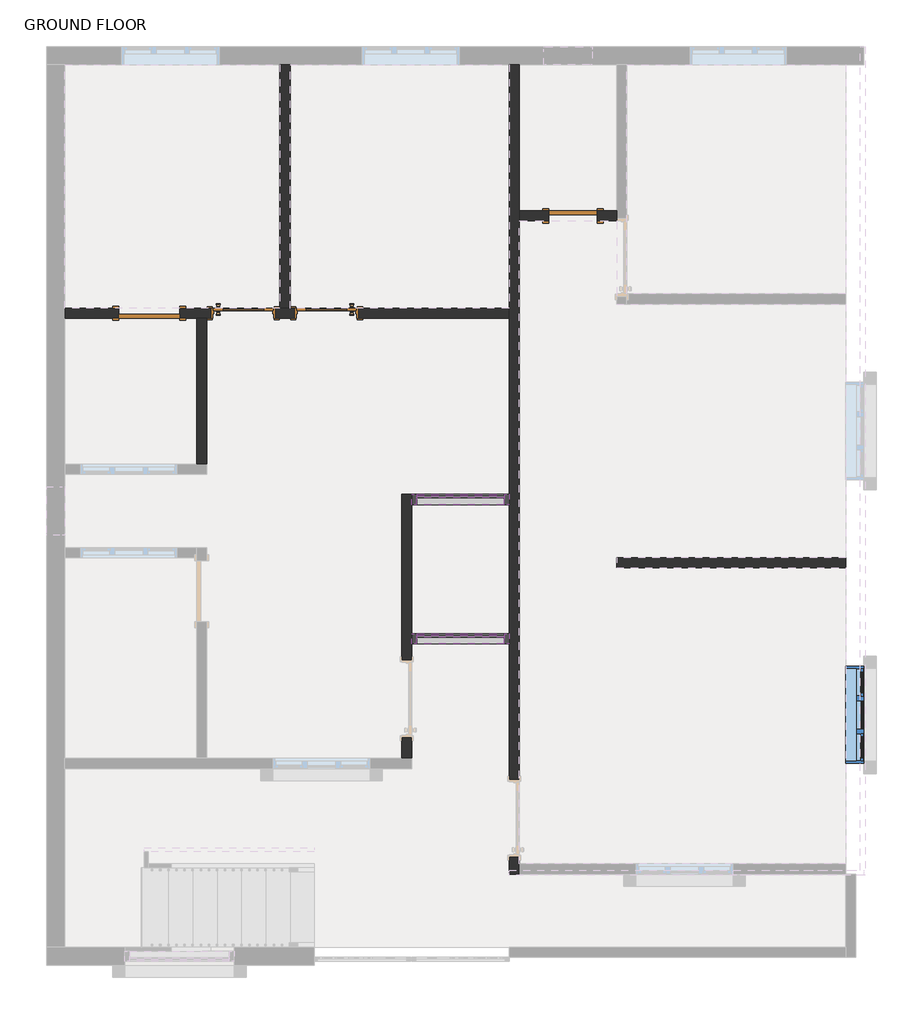
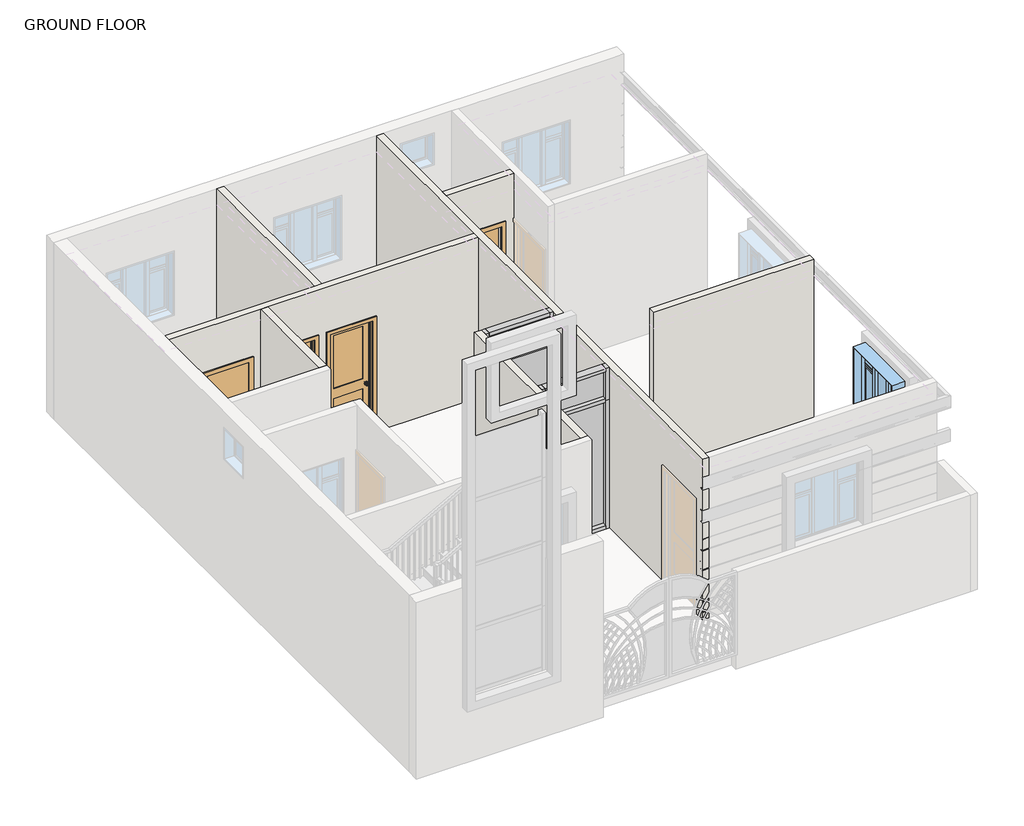
# One storey, part 3 of 7: 14 members, 7 walls, 4 doors, 4 plates, 1 window.
"""IFC4 building model written with IfcOpenShell, lengths in millimetres."""

from ifc_helpers import new_model, si_unit, frame, origin, place, context, project, spatial, polyline, circle_curve, outline, extrude, faceted_brep, transform, mapped, element, save
from ifc_brep_helpers import plane_surface, cylinder_surface, revolved_surface, advanced_brep
from components import door_interior_single_2_panel_wood_main_doors_a5f98f63, door_interior_single_2_panel_wood_main_doors_4d656947, single_flush_bathroom_flush_door_4d6c7550, single_flush_bathroom_flush_door_2_931cabab, member_273a15f2, member_867fe1e1, member_ee409385, member_47bfaf8a, system_panel_glazed_c5a9eb28, system_panel_glazed_3290db12, window_casement_triple_side_transom_window_4_x_4_fd24aed3

model = new_model("IFC4")

# Units and contexts
model_context = context("Model", 3, world=origin())
ifc_project = project(units=[si_unit("LENGTHUNIT", "METRE", prefix="MILLI")], contexts=[model_context])

# Site, building, storey
site = spatial("IfcSite", under=ifc_project)
building = spatial("IfcBuilding", under=site)
storey = spatial("IfcBuildingStorey", under=building, Name="GROUND FLOOR", Elevation=304.8)

# Doors
placement = place(None, origin())
door_interior_single_2_panel_wood_main_doors_shape = door_interior_single_2_panel_wood_main_doors_a5f98f63(model_context)
element("IfcDoor", 1, ObjectType="Door-Interior-Single-2_Panel-Wood : MAIN DOORS", at=placement, inside=storey, context=model_context, shape_type="MappedRepresentation", body=[
    mapped(door_interior_single_2_panel_wood_main_doors_shape, transform((-12525.5023867, 5183.9250137, 304.8), x_axis=(1.0, 0.0, 0.0), y_axis=(0.0, 1.0, 0.0), z_axis=(0.0, 0.0, 1.0))),
])
door_interior_single_2_panel_wood_main_doors_2_shape = door_interior_single_2_panel_wood_main_doors_4d656947(model_context)
element("IfcDoor", 2, ObjectType="Door-Interior-Single-2_Panel-Wood : MAIN DOORS", at=placement, inside=storey, context=model_context, shape_type="MappedRepresentation", body=[
    mapped(door_interior_single_2_panel_wood_main_doors_2_shape, transform((-11484.1023867, 5183.9250137, 304.8), x_axis=(-1.0, 0.0, 0.0), y_axis=(0.0, -1.0, 0.0), z_axis=(0.0, 0.0, 1.0))),
])
single_flush_bathroom_flush_door_shape = single_flush_bathroom_flush_door_4d6c7550(model_context)
element("IfcDoor", 3, ObjectType="Single-Flush : BATHROOM FLUSH DOOR", at=placement, inside=storey, context=model_context, shape_type="MappedRepresentation", body=[
    mapped(single_flush_bathroom_flush_door_shape, transform((-13706.6023867, 5180.7500137, 304.8), x_axis=(-1.0, 0.0, 0.0), y_axis=(0.0, -1.0, 0.0), z_axis=(0.0, 0.0, 1.0))),
])
single_flush_bathroom_flush_door_2_shape = single_flush_bathroom_flush_door_2_931cabab(model_context)
element("IfcDoor", 4, ObjectType="Single-Flush : BATHROOM FLUSH DOOR 2", at=placement, inside=storey, context=model_context, shape_type="MappedRepresentation", body=[
    mapped(single_flush_bathroom_flush_door_2_shape, transform((-8398.0023867, 6399.9500137, 304.8), x_axis=(-1.0, 0.0, 0.0), y_axis=(0.0, -1.0, 0.0), z_axis=(0.0, 0.0, 1.0))),
])

# Members
member_shape = member_273a15f2(model_context)
element("IfcMember", 5, ObjectType="Rectangular Mullion : 2.5\" x 5\" rectangular", at=placement, inside=storey, context=model_context, shape_type="MappedRepresentation", body=[
    mapped(member_shape, transform((-9261.6023867, 2848.1833471, 3352.8), x_axis=(0.0, 0.0, 1.0), y_axis=(0.0, -1.0, 0.0), z_axis=(1.0, 0.0, 0.0))),
])
element("IfcMember", 6, ObjectType="Rectangular Mullion : 2.5\" x 5\" rectangular", at=placement, inside=storey, context=model_context, shape_type="MappedRepresentation", body=[
    mapped(member_shape, transform((-9261.6023867, 1104.0500137, 3352.8), x_axis=(0.0, 0.0, 1.0), y_axis=(0.0, -1.0, 0.0), z_axis=(1.0, 0.0, 0.0))),
])
element("IfcMember", 7, ObjectType="Rectangular Mullion : 2.5\" x 5\" rectangular", at=placement, inside=storey, context=model_context, shape_type="MappedRepresentation", body=[
    mapped(member_shape, transform((-10353.8023867, 2848.1833471, 304.8), x_axis=(0.0, 0.0, -1.0), y_axis=(0.0, -1.0, 0.0), z_axis=(-1.0, 0.0, 0.0))),
])
element("IfcMember", 8, ObjectType="Rectangular Mullion : 2.5\" x 5\" rectangular", at=placement, inside=storey, context=model_context, shape_type="MappedRepresentation", body=[
    mapped(member_shape, transform((-10353.8023867, 1104.0500137, 304.8), x_axis=(0.0, 0.0, -1.0), y_axis=(0.0, -1.0, 0.0), z_axis=(-1.0, 0.0, 0.0))),
])
member_2_shape = member_867fe1e1(model_context)
element("IfcMember", 9, ObjectType="Rectangular Mullion : 2.5\" x 5\" rectangular", at=placement, inside=storey, context=model_context, shape_type="MappedRepresentation", body=[
    mapped(member_2_shape, transform((-9261.6023867, 2848.1833471, 2743.2), x_axis=(0.0, 0.0, 1.0), y_axis=(0.0, -1.0, 0.0), z_axis=(1.0, 0.0, 0.0))),
])
element("IfcMember", 10, ObjectType="Rectangular Mullion : 2.5\" x 5\" rectangular", at=placement, inside=storey, context=model_context, shape_type="MappedRepresentation", body=[
    mapped(member_2_shape, transform((-9261.6023867, 1104.0500137, 2743.2), x_axis=(0.0, 0.0, 1.0), y_axis=(0.0, -1.0, 0.0), z_axis=(1.0, 0.0, 0.0))),
])
member_3_shape = member_ee409385(model_context)
element("IfcMember", 11, ObjectType="Rectangular Mullion : 2.5\" x 5\" rectangular", at=placement, inside=storey, context=model_context, shape_type="MappedRepresentation", body=[
    mapped(member_3_shape, transform((-9198.1023867, 2848.1833471, 304.8), x_axis=(1.0, 0.0, 0.0), y_axis=(0.0, -1.0, 0.0), z_axis=(0.0, 0.0, -1.0))),
])
element("IfcMember", 12, ObjectType="Rectangular Mullion : 2.5\" x 5\" rectangular", at=placement, inside=storey, context=model_context, shape_type="MappedRepresentation", body=[
    mapped(member_3_shape, transform((-9198.1023867, 1104.0500137, 304.8), x_axis=(1.0, 0.0, 0.0), y_axis=(0.0, -1.0, 0.0), z_axis=(0.0, 0.0, -1.0))),
])
member_4_shape = member_47bfaf8a(model_context)
element("IfcMember", 13, ObjectType="Rectangular Mullion : 2.5\" x 5\" rectangular", at=placement, inside=storey, context=model_context, shape_type="MappedRepresentation", body=[
    mapped(member_4_shape, transform((-10417.3023867, 2848.1833471, 3352.8), x_axis=(-1.0, 0.0, 0.0), y_axis=(0.0, -1.0, 0.0), z_axis=(0.0, 0.0, 1.0))),
])
element("IfcMember", 14, ObjectType="Rectangular Mullion : 2.5\" x 5\" rectangular", at=placement, inside=storey, context=model_context, shape_type="MappedRepresentation", body=[
    mapped(member_4_shape, transform((-10417.3023867, 1104.0500137, 3352.8), x_axis=(-1.0, 0.0, 0.0), y_axis=(0.0, -1.0, 0.0), z_axis=(0.0, 0.0, 1.0))),
])
element("IfcMember", 15, ObjectType="Rectangular Mullion : 2.5\" x 5\" rectangular", at=placement, inside=storey, context=model_context, shape_type="MappedRepresentation", body=[
    mapped(member_4_shape, transform((-9198.1023867, 2848.1833471, 2743.2), x_axis=(1.0, 0.0, 0.0), y_axis=(0.0, -1.0, 0.0), z_axis=(0.0, 0.0, -1.0))),
])
element("IfcMember", 16, ObjectType="Rectangular Mullion : 2.5\" x 5\" rectangular", at=placement, inside=storey, context=model_context, shape_type="MappedRepresentation", body=[
    mapped(member_4_shape, transform((-9198.1023867, 1104.0500137, 2743.2), x_axis=(1.0, 0.0, 0.0), y_axis=(0.0, -1.0, 0.0), z_axis=(0.0, 0.0, -1.0))),
])
element("IfcMember", 17, ObjectType="Rectangular Mullion : 2.5\" x 5\" rectangular", at=placement, inside=storey, context=model_context, shape_type="MappedRepresentation", body=[
    mapped(member_3_shape, transform((-10417.3023867, 2848.1833471, 2743.2), x_axis=(-1.0, 0.0, 0.0), y_axis=(0.0, -1.0, 0.0), z_axis=(0.0, 0.0, 1.0))),
])
element("IfcMember", 18, ObjectType="Rectangular Mullion : 2.5\" x 5\" rectangular", at=placement, inside=storey, context=model_context, shape_type="MappedRepresentation", body=[
    mapped(member_3_shape, transform((-10417.3023867, 1104.0500137, 2743.2), x_axis=(-1.0, 0.0, 0.0), y_axis=(0.0, -1.0, 0.0), z_axis=(0.0, 0.0, 1.0))),
])

# Plates
system_panel_glazed_shape = system_panel_glazed_c5a9eb28(model_context)
element("IfcPlate", 19, ObjectType="System Panel : Glazed", at=placement, inside=storey, context=model_context, shape_type="MappedRepresentation", body=[
    mapped(system_panel_glazed_shape, transform((-9807.7023867, 2848.1833471, 368.3), x_axis=(1.0, 0.0, 0.0), y_axis=(0.0, 1.0, 0.0), z_axis=(0.0, 0.0, 1.0))),
])
element("IfcPlate", 20, ObjectType="System Panel : Glazed", at=placement, inside=storey, context=model_context, shape_type="MappedRepresentation", body=[
    mapped(system_panel_glazed_shape, transform((-9807.7023867, 1104.0500137, 368.3), x_axis=(1.0, 0.0, 0.0), y_axis=(0.0, 1.0, 0.0), z_axis=(0.0, 0.0, 1.0))),
])
system_panel_glazed_2_shape = system_panel_glazed_3290db12(model_context)
element("IfcPlate", 21, ObjectType="System Panel : Glazed", at=placement, inside=storey, context=model_context, shape_type="MappedRepresentation", body=[
    mapped(system_panel_glazed_2_shape, transform((-9807.7023867, 2848.1833471, 2774.95), x_axis=(1.0, 0.0, 0.0), y_axis=(0.0, 1.0, 0.0), z_axis=(0.0, 0.0, 1.0))),
])
element("IfcPlate", 22, ObjectType="System Panel : Glazed", at=placement, inside=storey, context=model_context, shape_type="MappedRepresentation", body=[
    mapped(system_panel_glazed_2_shape, transform((-9807.7023867, 1104.0500137, 2774.95), x_axis=(1.0, 0.0, 0.0), y_axis=(0.0, 1.0, 0.0), z_axis=(0.0, 0.0, 1.0))),
])

# Walls
element("IfcWall", 23, ObjectType="INNER WALL 5\"", at=placement, inside=storey, context=model_context, shape_type="AdvancedBrep", body=[
    advanced_brep(
    [(-9198.1023867, -1842.3499863, 3352.8), (-9198.1023867, 5117.2500137, 3352.8), (-9198.1023867, 5244.2500137, 3352.8), (-9198.1023867, 8292.2500137, 3352.8), (-9198.1023867, 8292.2500137, 304.8), (-9198.1023867, 5244.2500137, 304.8), (-9198.1023867, 5117.2500137, 304.8), (-9198.1023867, -661.2499863, 304.8), (-9198.1023867, -661.2499863, 2463.8), (-9198.1023867, -1626.4499863, 2463.8), (-9198.1023867, -1626.4499863, 304.8), (-9198.1023867, -1842.3499863, 304.8), (-9198.1023867, -1842.3499863, 444.5), (-9198.1023867, -1793.9883863, 444.5), (-9198.1023867, -1793.9883863, 445.8796758), (-9198.1023867, -1798.3711955, 451.0534103), (-9198.1023867, -1821.9918863, 454.9902), (-9198.1023867, -1841.2297679, 458.19652), (-9198.1023867, -1842.3499863, 458.44689), (-9198.1023867, -1842.3499863, 659.15311), (-9198.1023867, -1841.2297679, 659.40348), (-9198.1023867, -1821.9918863, 662.6098), (-9198.1023867, -1798.3711955, 666.5465897), (-9198.1023867, -1793.9883863, 671.7203242), (-9198.1023867, -1793.9883863, 673.1), (-9198.1023867, -1842.3499863, 673.1), (-9198.1023867, -1842.3499863, 1028.7), (-9198.1023867, -1793.9883863, 1028.7), (-9198.1023867, -1793.9883863, 1030.0796758), (-9198.1023867, -1798.3711955, 1035.2534103), (-9198.1023867, -1821.9918863, 1039.1902), (-9198.1023867, -1841.2297679, 1042.39652), (-9198.1023867, -1842.3499863, 1042.64689), (-9198.1023867, -1842.3499863, 1243.35311), (-9198.1023867, -1841.2297679, 1243.60348), (-9198.1023867, -1821.9918863, 1246.8098), (-9198.1023867, -1798.3711955, 1250.7465897), (-9198.1023867, -1793.9883863, 1255.9203242), (-9198.1023867, -1793.9883863, 1257.3), (-9198.1023867, -1842.3499863, 1257.3), (-9198.1023867, -1842.3499863, 1612.9), (-9198.1023867, -1793.9883863, 1612.9), (-9198.1023867, -1793.9883863, 1614.2796758), (-9198.1023867, -1798.3711955, 1619.4534103), (-9198.1023867, -1821.9918863, 1623.3902), (-9198.1023867, -1841.2297679, 1626.59652), (-9198.1023867, -1842.3499863, 1626.84689), (-9198.1023867, -1842.3499863, 1827.55311), (-9198.1023867, -1841.2297679, 1827.80348), (-9198.1023867, -1821.9918863, 1831.0098), (-9198.1023867, -1798.3711955, 1834.9465897), (-9198.1023867, -1793.9883863, 1840.1203242), (-9198.1023867, -1793.9883863, 1841.5), (-9198.1023867, -1842.3499863, 1841.5), (-9198.1023867, -1842.3499863, 2146.3), (-9198.1023867, -1793.9883863, 2146.3), (-9198.1023867, -1793.9883863, 2147.6796758), (-9198.1023867, -1798.3711955, 2152.8534103), (-9198.1023867, -1821.9918863, 2156.7902), (-9198.1023867, -1841.2297679, 2159.99652), (-9198.1023867, -1842.3499863, 2160.24689), (-9198.1023867, -1842.3499863, 2360.95311), (-9198.1023867, -1841.2297679, 2361.20348), (-9198.1023867, -1821.9918863, 2364.4098), (-9198.1023867, -1798.3711955, 2368.3465897), (-9198.1023867, -1793.9883863, 2373.5203242), (-9198.1023867, -1793.9883863, 2374.9), (-9198.1023867, -1842.3499863, 2374.9), (-9198.1023867, -1842.3499863, 2781.3), (-9198.1023867, -1793.9883863, 2781.3), (-9198.1023867, -1793.9883863, 2782.6796758), (-9198.1023867, -1798.3711955, 2787.8534103), (-9198.1023867, -1821.9918863, 2791.7902), (-9198.1023867, -1841.2297679, 2794.99652), (-9198.1023867, -1842.3499863, 2795.24689), (-9198.1023867, -1842.3499863, 2995.95311), (-9198.1023867, -1841.2297679, 2996.20348), (-9198.1023867, -1821.9918863, 2999.4098), (-9198.1023867, -1798.3711955, 3003.3465897), (-9198.1023867, -1793.9883863, 3008.5203242), (-9198.1023867, -1793.9883863, 3009.9), (-9198.1023867, -1842.3499863, 3009.9), (-9071.1023867, 8292.2500137, 3352.8), (-9071.1023867, 6463.4500137, 3352.8), (-9071.1023867, 6336.4500137, 3352.8), (-9071.1023867, -1715.3499863, 3352.8), (-9071.1023867, -1842.3499863, 3352.8), (-9071.1023867, -1842.3499863, 3009.9), (-9071.1023867, -1793.9883863, 3009.9), (-9071.1023867, -1793.9883863, 3008.5203242), (-9071.1023867, -1798.3711955, 3003.3465897), (-9071.1023867, -1821.9918863, 2999.4098), (-9071.1023867, -1841.2297679, 2996.20348), (-9071.1023867, -1842.3499863, 2995.95311), (-9071.1023867, -1842.3499863, 2795.24689), (-9071.1023867, -1841.2297679, 2794.99652), (-9071.1023867, -1821.9918863, 2791.7902), (-9071.1023867, -1798.3711955, 2787.8534103), (-9071.1023867, -1793.9883863, 2782.6796758), (-9071.1023867, -1793.9883863, 2781.3), (-9071.1023867, -1842.3499863, 2781.3), (-9071.1023867, -1842.3499863, 2374.9), (-9071.1023867, -1793.9883863, 2374.9), (-9071.1023867, -1793.9883863, 2373.5203242), (-9071.1023867, -1798.3711955, 2368.3465897), (-9071.1023867, -1821.9918863, 2364.4098), (-9071.1023867, -1841.2297679, 2361.20348), (-9071.1023867, -1842.3499863, 2360.95311), (-9071.1023867, -1842.3499863, 2160.24689), (-9071.1023867, -1841.2297679, 2159.99652), (-9071.1023867, -1821.9918863, 2156.7902), (-9071.1023867, -1798.3711955, 2152.8534103), (-9071.1023867, -1793.9883863, 2147.6796758), (-9071.1023867, -1793.9883863, 2146.3), (-9071.1023867, -1842.3499863, 2146.3), (-9071.1023867, -1842.3499863, 1841.5), (-9071.1023867, -1793.9883863, 1841.5), (-9071.1023867, -1793.9883863, 1840.1203242), (-9071.1023867, -1798.3711955, 1834.9465897), (-9071.1023867, -1821.9918863, 1831.0098), (-9071.1023867, -1841.2297679, 1827.80348), (-9071.1023867, -1842.3499863, 1827.55311), (-9071.1023867, -1842.3499863, 1626.84689), (-9071.1023867, -1841.2297679, 1626.59652), (-9071.1023867, -1821.9918863, 1623.3902), (-9071.1023867, -1798.3711955, 1619.4534103), (-9071.1023867, -1793.9883863, 1614.2796758), (-9071.1023867, -1793.9883863, 1612.9), (-9071.1023867, -1842.3499863, 1612.9), (-9071.1023867, -1842.3499863, 1257.3), (-9071.1023867, -1793.9883863, 1257.3), (-9071.1023867, -1793.9883863, 1255.9203242), (-9071.1023867, -1798.3711955, 1250.7465897), (-9071.1023867, -1821.9918863, 1246.8098), (-9071.1023867, -1841.2297679, 1243.60348), (-9071.1023867, -1842.3499863, 1243.35311), (-9071.1023867, -1842.3499863, 1042.64689), (-9071.1023867, -1841.2297679, 1042.39652), (-9071.1023867, -1821.9918863, 1039.1902), (-9071.1023867, -1798.3711955, 1035.2534103), (-9071.1023867, -1793.9883863, 1030.0796758), (-9071.1023867, -1793.9883863, 1028.7), (-9071.1023867, -1842.3499863, 1028.7), (-9071.1023867, -1842.3499863, 673.1), (-9071.1023867, -1793.9883863, 673.1), (-9071.1023867, -1793.9883863, 671.7203242), (-9071.1023867, -1798.3711955, 666.5465897), (-9071.1023867, -1821.9918863, 662.6098), (-9071.1023867, -1841.2297679, 659.40348), (-9071.1023867, -1842.3499863, 659.15311), (-9071.1023867, -1842.3499863, 458.44689), (-9071.1023867, -1841.2297679, 458.19652), (-9071.1023867, -1821.9918863, 454.9902), (-9071.1023867, -1798.3711955, 451.0534103), (-9071.1023867, -1793.9883863, 445.8796758), (-9071.1023867, -1793.9883863, 444.5), (-9071.1023867, -1842.3499863, 444.5), (-9071.1023867, -1842.3499863, 304.8), (-9071.1023867, -1626.4499863, 304.8), (-9071.1023867, -1626.4499863, 2463.8), (-9071.1023867, -661.2499863, 2463.8), (-9071.1023867, -661.2499863, 304.8), (-9071.1023867, 6336.4500137, 304.8), (-9071.1023867, 6463.4500137, 304.8), (-9071.1023867, 8292.2500137, 304.8)],
    [
        (0, 1),
        (1, 2),
        (2, 3),
        (3, 4),
        (4, 5),
        (5, 6),
        (6, 7),
        (7, 8),
        (8, 9),
        (9, 10),
        (10, 11),
        (11, 12),
        (12, 13),
        (13, 14),
        (14, 15, circle_curve(frame((-9198.1023867, -1799.2334863, 445.8796758), z_axis=(1.0, 0.0, 0.0), x_axis=(0.0, 1.0, 0.0)), 5.2451)),
        (15, 16),
        (16, 17),
        (17, 18, circle_curve(frame((-9198.1023867, -1839.5051863, 468.543989), z_axis=(-1.0, 0.0, 0.0), x_axis=(0.0, 1.0, 0.0)), 10.4902)),
        (18, 19),
        (19, 20, circle_curve(frame((-9198.1023867, -1839.5051863, 649.056011), z_axis=(-1.0, 0.0, 0.0), x_axis=(0.0, 1.0, 0.0)), 10.4902)),
        (20, 21),
        (21, 22),
        (22, 23, circle_curve(frame((-9198.1023867, -1799.2334863, 671.7203242), z_axis=(1.0, 0.0, 0.0), x_axis=(0.0, 1.0, 0.0)), 5.2451)),
        (23, 24),
        (24, 25),
        (25, 26),
        (26, 27),
        (27, 28),
        (28, 29, circle_curve(frame((-9198.1023867, -1799.2334863, 1030.0796758), z_axis=(1.0, 0.0, 0.0), x_axis=(0.0, 1.0, 0.0)), 5.2451)),
        (29, 30),
        (30, 31),
        (31, 32, circle_curve(frame((-9198.1023867, -1839.5051863, 1052.743989), z_axis=(-1.0, 0.0, 0.0), x_axis=(0.0, 1.0, 0.0)), 10.4902)),
        (32, 33),
        (33, 34, circle_curve(frame((-9198.1023867, -1839.5051863, 1233.256011), z_axis=(-1.0, 0.0, 0.0), x_axis=(0.0, 1.0, 0.0)), 10.4902)),
        (34, 35),
        (35, 36),
        (36, 37, circle_curve(frame((-9198.1023867, -1799.2334863, 1255.9203242), z_axis=(1.0, 0.0, 0.0), x_axis=(0.0, 1.0, 0.0)), 5.2451)),
        (37, 38),
        (38, 39),
        (39, 40),
        (40, 41),
        (41, 42),
        (42, 43, circle_curve(frame((-9198.1023867, -1799.2334863, 1614.2796758), z_axis=(1.0, 0.0, 0.0), x_axis=(0.0, 1.0, 0.0)), 5.2451)),
        (43, 44),
        (44, 45),
        (45, 46, circle_curve(frame((-9198.1023867, -1839.5051863, 1636.943989), z_axis=(-1.0, 0.0, 0.0), x_axis=(0.0, 1.0, 0.0)), 10.4902)),
        (46, 47),
        (47, 48, circle_curve(frame((-9198.1023867, -1839.5051863, 1817.456011), z_axis=(-1.0, 0.0, 0.0), x_axis=(0.0, 1.0, 0.0)), 10.4902)),
        (48, 49),
        (49, 50),
        (50, 51, circle_curve(frame((-9198.1023867, -1799.2334863, 1840.1203242), z_axis=(1.0, 0.0, 0.0), x_axis=(0.0, 1.0, 0.0)), 5.2451)),
        (51, 52),
        (52, 53),
        (53, 54),
        (54, 55),
        (55, 56),
        (56, 57, circle_curve(frame((-9198.1023867, -1799.2334863, 2147.6796758), z_axis=(1.0, 0.0, 0.0), x_axis=(0.0, 1.0, 0.0)), 5.2451)),
        (57, 58),
        (58, 59),
        (59, 60, circle_curve(frame((-9198.1023867, -1839.5051863, 2170.343989), z_axis=(-1.0, 0.0, 0.0), x_axis=(0.0, 1.0, 0.0)), 10.4902)),
        (60, 61),
        (61, 62, circle_curve(frame((-9198.1023867, -1839.5051863, 2350.856011), z_axis=(-1.0, 0.0, 0.0), x_axis=(0.0, 1.0, 0.0)), 10.4902)),
        (62, 63),
        (63, 64),
        (64, 65, circle_curve(frame((-9198.1023867, -1799.2334863, 2373.5203242), z_axis=(1.0, 0.0, 0.0), x_axis=(0.0, 1.0, 0.0)), 5.2451)),
        (65, 66),
        (66, 67),
        (67, 68),
        (68, 69),
        (69, 70),
        (70, 71, circle_curve(frame((-9198.1023867, -1799.2334863, 2782.6796758), z_axis=(1.0, 0.0, 0.0), x_axis=(0.0, 1.0, 0.0)), 5.2451)),
        (71, 72),
        (72, 73),
        (73, 74, circle_curve(frame((-9198.1023867, -1839.5051863, 2805.343989), z_axis=(-1.0, 0.0, 0.0), x_axis=(0.0, 1.0, 0.0)), 10.4902)),
        (74, 75),
        (75, 76, circle_curve(frame((-9198.1023867, -1839.5051863, 2985.856011), z_axis=(-1.0, 0.0, 0.0), x_axis=(0.0, 1.0, 0.0)), 10.4902)),
        (76, 77),
        (77, 78),
        (78, 79, circle_curve(frame((-9198.1023867, -1799.2334863, 3008.5203242), z_axis=(1.0, 0.0, 0.0), x_axis=(0.0, 1.0, 0.0)), 5.2451)),
        (79, 80),
        (80, 81),
        (81, 0),
        (82, 83),
        (83, 84),
        (84, 85),
        (85, 86),
        (86, 87),
        (87, 88),
        (88, 89),
        (89, 90, circle_curve(frame((-9071.1023867, -1799.2334863, 3008.5203242), z_axis=(-1.0, 0.0, 0.0), x_axis=(0.0, 1.0, 0.0)), 5.2451)),
        (90, 91),
        (91, 92),
        (92, 93, circle_curve(frame((-9071.1023867, -1839.5051863, 2985.856011), z_axis=(1.0, 0.0, 0.0), x_axis=(0.0, 1.0, 0.0)), 10.4902)),
        (93, 94),
        (94, 95, circle_curve(frame((-9071.1023867, -1839.5051863, 2805.343989), z_axis=(1.0, 0.0, 0.0), x_axis=(0.0, 1.0, 0.0)), 10.4902)),
        (95, 96),
        (96, 97),
        (97, 98, circle_curve(frame((-9071.1023867, -1799.2334863, 2782.6796758), z_axis=(-1.0, 0.0, 0.0), x_axis=(0.0, 1.0, 0.0)), 5.2451)),
        (98, 99),
        (99, 100),
        (100, 101),
        (101, 102),
        (102, 103),
        (103, 104, circle_curve(frame((-9071.1023867, -1799.2334863, 2373.5203242), z_axis=(-1.0, 0.0, 0.0), x_axis=(0.0, 1.0, 0.0)), 5.2451)),
        (104, 105),
        (105, 106),
        (106, 107, circle_curve(frame((-9071.1023867, -1839.5051863, 2350.856011), z_axis=(1.0, 0.0, 0.0), x_axis=(0.0, 1.0, 0.0)), 10.4902)),
        (107, 108),
        (108, 109, circle_curve(frame((-9071.1023867, -1839.5051863, 2170.343989), z_axis=(1.0, 0.0, 0.0), x_axis=(0.0, 1.0, 0.0)), 10.4902)),
        (109, 110),
        (110, 111),
        (111, 112, circle_curve(frame((-9071.1023867, -1799.2334863, 2147.6796758), z_axis=(-1.0, 0.0, 0.0), x_axis=(0.0, 1.0, 0.0)), 5.2451)),
        (112, 113),
        (113, 114),
        (114, 115),
        (115, 116),
        (116, 117),
        (117, 118, circle_curve(frame((-9071.1023867, -1799.2334863, 1840.1203242), z_axis=(-1.0, 0.0, 0.0), x_axis=(0.0, 1.0, 0.0)), 5.2451)),
        (118, 119),
        (119, 120),
        (120, 121, circle_curve(frame((-9071.1023867, -1839.5051863, 1817.456011), z_axis=(1.0, 0.0, 0.0), x_axis=(0.0, 1.0, 0.0)), 10.4902)),
        (121, 122),
        (122, 123, circle_curve(frame((-9071.1023867, -1839.5051863, 1636.943989), z_axis=(1.0, 0.0, 0.0), x_axis=(0.0, 1.0, 0.0)), 10.4902)),
        (123, 124),
        (124, 125),
        (125, 126, circle_curve(frame((-9071.1023867, -1799.2334863, 1614.2796758), z_axis=(-1.0, 0.0, 0.0), x_axis=(0.0, 1.0, 0.0)), 5.2451)),
        (126, 127),
        (127, 128),
        (128, 129),
        (129, 130),
        (130, 131),
        (131, 132, circle_curve(frame((-9071.1023867, -1799.2334863, 1255.9203242), z_axis=(-1.0, 0.0, 0.0), x_axis=(0.0, 1.0, 0.0)), 5.2451)),
        (132, 133),
        (133, 134),
        (134, 135, circle_curve(frame((-9071.1023867, -1839.5051863, 1233.256011), z_axis=(1.0, 0.0, 0.0), x_axis=(0.0, 1.0, 0.0)), 10.4902)),
        (135, 136),
        (136, 137, circle_curve(frame((-9071.1023867, -1839.5051863, 1052.743989), z_axis=(1.0, 0.0, 0.0), x_axis=(0.0, 1.0, 0.0)), 10.4902)),
        (137, 138),
        (138, 139),
        (139, 140, circle_curve(frame((-9071.1023867, -1799.2334863, 1030.0796758), z_axis=(-1.0, 0.0, 0.0), x_axis=(0.0, 1.0, 0.0)), 5.2451)),
        (140, 141),
        (141, 142),
        (142, 143),
        (143, 144),
        (144, 145),
        (145, 146, circle_curve(frame((-9071.1023867, -1799.2334863, 671.7203242), z_axis=(-1.0, 0.0, 0.0), x_axis=(0.0, 1.0, 0.0)), 5.2451)),
        (146, 147),
        (147, 148),
        (148, 149, circle_curve(frame((-9071.1023867, -1839.5051863, 649.056011), z_axis=(1.0, 0.0, 0.0), x_axis=(0.0, 1.0, 0.0)), 10.4902)),
        (149, 150),
        (150, 151, circle_curve(frame((-9071.1023867, -1839.5051863, 468.543989), z_axis=(1.0, 0.0, 0.0), x_axis=(0.0, 1.0, 0.0)), 10.4902)),
        (151, 152),
        (152, 153),
        (153, 154, circle_curve(frame((-9071.1023867, -1799.2334863, 445.8796758), z_axis=(-1.0, 0.0, 0.0), x_axis=(0.0, 1.0, 0.0)), 5.2451)),
        (154, 155),
        (155, 156),
        (156, 157),
        (157, 158),
        (158, 159),
        (159, 160),
        (160, 161),
        (161, 162),
        (162, 163),
        (163, 164),
        (164, 82),
        (4, 164),
        (161, 7),
        (157, 11),
        (10, 158),
        (0, 86),
        (82, 3),
        (156, 12),
        (81, 87),
        (74, 94),
        (93, 75),
        (100, 68),
        (67, 101),
        (25, 143),
        (142, 26),
        (149, 19),
        (18, 150),
        (39, 129),
        (128, 40),
        (135, 33),
        (32, 136),
        (53, 115),
        (114, 54),
        (121, 47),
        (46, 122),
        (60, 108),
        (107, 61),
        (160, 8),
        (159, 9),
        (80, 88),
        (79, 89),
        (78, 90),
        (77, 91),
        (76, 92),
        (73, 95),
        (72, 96),
        (71, 97),
        (70, 98),
        (69, 99),
        (24, 144),
        (23, 145),
        (22, 146),
        (21, 147),
        (20, 148),
        (17, 151),
        (16, 152),
        (15, 153),
        (14, 154),
        (13, 155),
        (38, 130),
        (37, 131),
        (36, 132),
        (35, 133),
        (34, 134),
        (31, 137),
        (30, 138),
        (29, 139),
        (28, 140),
        (27, 141),
        (52, 116),
        (51, 117),
        (50, 118),
        (49, 119),
        (48, 120),
        (45, 123),
        (44, 124),
        (43, 125),
        (42, 126),
        (41, 127),
        (66, 102),
        (65, 103),
        (64, 104),
        (63, 105),
        (62, 106),
        (59, 109),
        (58, 110),
        (57, 111),
        (56, 112),
        (55, 113),
    ],
    [
        plane_surface(frame((-9198.1023867, 8292.2500137, 304.8), z_axis=(-1.0, 0.0, 0.0), x_axis=(0.0, -1.0, 0.0))),
        plane_surface(frame((-9071.1023867, 8292.2500137, 304.8), z_axis=(1.0, 0.0, 0.0), x_axis=(0.0, 1.0, 0.0))),
        plane_surface(frame((-9198.1023867, 8406.5500137, 304.8), z_axis=(0.0, 0.0, -1.0), x_axis=(1.0, 0.0, 0.0))),
        plane_surface(frame((-9198.1023867, -1778.8499863, 3352.8), z_axis=(0.0, 0.0, 1.0), x_axis=(1.0, 0.0, 0.0))),
        plane_surface(frame((-14983.6015581, 8292.2500137, 0.0), z_axis=(0.0, 1.0, 0.0), x_axis=(1.0, 0.0, 0.0))),
        plane_surface(frame((-9198.1023867, -1842.3499863, 0.0), z_axis=(0.0, -1.0, 0.0), x_axis=(1.0, 0.0, 0.0))),
        plane_surface(frame((-7674.1023867, -661.2499863, 304.8), z_axis=(0.0, -1.0, 0.0), x_axis=(-1.0, 0.0, 0.0))),
        plane_surface(frame((-7674.1023867, -661.2499863, 2463.8), z_axis=(0.0, 0.0, -1.0), x_axis=(-1.0, 0.0, 0.0))),
        plane_surface(frame((-7674.1023867, -1626.4499863, 2463.8), z_axis=(0.0, 1.0, 0.0), x_axis=(-1.0, 0.0, 0.0))),
        plane_surface(frame((-9198.1023867, -1857.2343863, 3009.9), z_axis=(0.0, 0.0, -1.0), x_axis=(1.0, 0.0, 0.0))),
        plane_surface(frame((-9198.1023867, -1793.9883863, 3009.9), z_axis=(0.0, -1.0, 0.0), x_axis=(1.0, 0.0, 0.0))),
        revolved_surface(polyline([(-9198.1023867, -1793.9883863, 3008.5203242), (-9071.1023867, -1793.9883863, 3008.5203242)]), (-9198.1023867, -1799.2334863, 3008.5203242), (-1.0, 0.0, 0.0)),
        plane_surface(frame((-9198.1023867, -1798.3711955, 3003.3465897), z_axis=(0.0, -0.16439930721687082, 0.9863938705135049), x_axis=(1.0, 0.0, 0.0))),
        plane_surface(frame((-9198.1023867, -1821.9918863, 2999.4098), z_axis=(0.0, -0.16439930721687146, 0.9863938705135048), x_axis=(1.0, 0.0, 0.0))),
        cylinder_surface(frame((-9198.1023867, -1839.5051863, 2985.856011), z_axis=(1.0, 0.0, 0.0), x_axis=(0.0, 1.0, 0.0)), 10.4902),
        cylinder_surface(frame((-9198.1023867, -1839.5051863, 2805.343989), z_axis=(1.0, 0.0, 0.0), x_axis=(0.0, 1.0, 0.0)), 10.4902),
        plane_surface(frame((-9198.1023867, -1841.2297679, 2794.99652), z_axis=(0.0, -0.1643993072168769, -0.9863938705135039), x_axis=(1.0, 0.0, 0.0))),
        plane_surface(frame((-9198.1023867, -1821.9918863, 2791.7902), z_axis=(0.0, -0.16439930721687793, -0.9863938705135037), x_axis=(1.0, 0.0, 0.0))),
        revolved_surface(polyline([(-9198.1023867, -1793.9883863, 2782.6796758), (-9071.1023867, -1793.9883863, 2782.6796758)]), (-9198.1023867, -1799.2334863, 2782.6796758), (-1.0, 0.0, 0.0)),
        plane_surface(frame((-9198.1023867, -1793.9883863, 2782.6796758), z_axis=(0.0, -1.0, 0.0), x_axis=(1.0, 0.0, 0.0))),
        plane_surface(frame((-9198.1023867, -1793.9883863, 2781.3), z_axis=(0.0, 0.0, 1.0), x_axis=(1.0, 0.0, 0.0))),
        plane_surface(frame((-9198.1023867, -1857.2343863, 673.1), z_axis=(0.0, 0.0, -1.0), x_axis=(1.0, 0.0, 0.0))),
        plane_surface(frame((-9198.1023867, -1793.9883863, 673.1), z_axis=(0.0, -1.0, 0.0), x_axis=(1.0, 0.0, 0.0))),
        revolved_surface(polyline([(-9198.1023867, -1793.9883863, 671.7203242), (-9071.1023867, -1793.9883863, 671.7203242)]), (-9198.1023867, -1799.2334863, 671.7203242), (-1.0, 0.0, 0.0)),
        plane_surface(frame((-9198.1023867, -1798.3711955, 666.5465897), z_axis=(0.0, -0.16439930721687082, 0.9863938705135049), x_axis=(1.0, 0.0, 0.0))),
        plane_surface(frame((-9198.1023867, -1821.9918863, 662.6098), z_axis=(0.0, -0.16439930721687146, 0.9863938705135048), x_axis=(1.0, 0.0, 0.0))),
        cylinder_surface(frame((-9198.1023867, -1839.5051863, 649.056011), z_axis=(1.0, 0.0, 0.0), x_axis=(0.0, 1.0, 0.0)), 10.4902),
        cylinder_surface(frame((-9198.1023867, -1839.5051863, 468.543989), z_axis=(1.0, 0.0, 0.0), x_axis=(0.0, 1.0, 0.0)), 10.4902),
        plane_surface(frame((-9198.1023867, -1841.2297679, 458.19652), z_axis=(0.0, -0.1643993072168769, -0.9863938705135039), x_axis=(1.0, 0.0, 0.0))),
        plane_surface(frame((-9198.1023867, -1821.9918863, 454.9902), z_axis=(0.0, -0.16439930721687793, -0.9863938705135037), x_axis=(1.0, 0.0, 0.0))),
        revolved_surface(polyline([(-9198.1023867, -1793.9883863, 445.8796758), (-9071.1023867, -1793.9883863, 445.8796758)]), (-9198.1023867, -1799.2334863, 445.8796758), (-1.0, 0.0, 0.0)),
        plane_surface(frame((-9198.1023867, -1793.9883863, 445.8796758), z_axis=(0.0, -1.0, 0.0), x_axis=(1.0, 0.0, 0.0))),
        plane_surface(frame((-9198.1023867, -1793.9883863, 444.5), z_axis=(0.0, 0.0, 1.0), x_axis=(1.0, 0.0, 0.0))),
        plane_surface(frame((-9198.1023867, -1857.2343863, 1257.3), z_axis=(0.0, 0.0, -1.0), x_axis=(1.0, 0.0, 0.0))),
        plane_surface(frame((-9198.1023867, -1793.9883863, 1257.3), z_axis=(0.0, -1.0, 0.0), x_axis=(1.0, 0.0, 0.0))),
        revolved_surface(polyline([(-9198.1023867, -1793.9883863, 1255.9203242), (-9071.1023867, -1793.9883863, 1255.9203242)]), (-9198.1023867, -1799.2334863, 1255.9203242), (-1.0, 0.0, 0.0)),
        plane_surface(frame((-9198.1023867, -1798.3711955, 1250.7465897), z_axis=(0.0, -0.16439930721687082, 0.9863938705135049), x_axis=(1.0, 0.0, 0.0))),
        plane_surface(frame((-9198.1023867, -1821.9918863, 1246.8098), z_axis=(0.0, -0.16439930721687146, 0.9863938705135048), x_axis=(1.0, 0.0, 0.0))),
        cylinder_surface(frame((-9198.1023867, -1839.5051863, 1233.256011), z_axis=(1.0, 0.0, 0.0), x_axis=(0.0, 1.0, 0.0)), 10.4902),
        cylinder_surface(frame((-9198.1023867, -1839.5051863, 1052.743989), z_axis=(1.0, 0.0, 0.0), x_axis=(0.0, 1.0, 0.0)), 10.4902),
        plane_surface(frame((-9198.1023867, -1841.2297679, 1042.39652), z_axis=(0.0, -0.1643993072168769, -0.9863938705135039), x_axis=(1.0, 0.0, 0.0))),
        plane_surface(frame((-9198.1023867, -1821.9918863, 1039.1902), z_axis=(0.0, -0.16439930721687793, -0.9863938705135037), x_axis=(1.0, 0.0, 0.0))),
        revolved_surface(polyline([(-9198.1023867, -1793.9883863, 1030.0796758), (-9071.1023867, -1793.9883863, 1030.0796758)]), (-9198.1023867, -1799.2334863, 1030.0796758), (-1.0, 0.0, 0.0)),
        plane_surface(frame((-9198.1023867, -1793.9883863, 1030.0796758), z_axis=(0.0, -1.0, 0.0), x_axis=(1.0, 0.0, 0.0))),
        plane_surface(frame((-9198.1023867, -1793.9883863, 1028.7), z_axis=(0.0, 0.0, 1.0), x_axis=(1.0, 0.0, 0.0))),
        plane_surface(frame((-9198.1023867, -1857.2343863, 1841.5), z_axis=(0.0, 0.0, -1.0), x_axis=(1.0, 0.0, 0.0))),
        plane_surface(frame((-9198.1023867, -1793.9883863, 1841.5), z_axis=(0.0, -1.0, 0.0), x_axis=(1.0, 0.0, 0.0))),
        revolved_surface(polyline([(-9198.1023867, -1793.9883863, 1840.1203242), (-9071.1023867, -1793.9883863, 1840.1203242)]), (-9198.1023867, -1799.2334863, 1840.1203242), (-1.0, 0.0, 0.0)),
        plane_surface(frame((-9198.1023867, -1798.3711955, 1834.9465897), z_axis=(0.0, -0.16439930721687082, 0.9863938705135049), x_axis=(1.0, 0.0, 0.0))),
        plane_surface(frame((-9198.1023867, -1821.9918863, 1831.0098), z_axis=(0.0, -0.16439930721687146, 0.9863938705135048), x_axis=(1.0, 0.0, 0.0))),
        cylinder_surface(frame((-9198.1023867, -1839.5051863, 1817.456011), z_axis=(1.0, 0.0, 0.0), x_axis=(0.0, 1.0, 0.0)), 10.4902),
        cylinder_surface(frame((-9198.1023867, -1839.5051863, 1636.943989), z_axis=(1.0, 0.0, 0.0), x_axis=(0.0, 1.0, 0.0)), 10.4902),
        plane_surface(frame((-9198.1023867, -1841.2297679, 1626.59652), z_axis=(0.0, -0.1643993072168769, -0.9863938705135039), x_axis=(1.0, 0.0, 0.0))),
        plane_surface(frame((-9198.1023867, -1821.9918863, 1623.3902), z_axis=(0.0, -0.16439930721687793, -0.9863938705135037), x_axis=(1.0, 0.0, 0.0))),
        revolved_surface(polyline([(-9198.1023867, -1793.9883863, 1614.2796758), (-9071.1023867, -1793.9883863, 1614.2796758)]), (-9198.1023867, -1799.2334863, 1614.2796758), (-1.0, 0.0, 0.0)),
        plane_surface(frame((-9198.1023867, -1793.9883863, 1614.2796758), z_axis=(0.0, -1.0, 0.0), x_axis=(1.0, 0.0, 0.0))),
        plane_surface(frame((-9198.1023867, -1793.9883863, 1612.9), z_axis=(0.0, 0.0, 1.0), x_axis=(1.0, 0.0, 0.0))),
        plane_surface(frame((-9198.1023867, -1857.2343863, 2374.9), z_axis=(0.0, 0.0, -1.0), x_axis=(1.0, 0.0, 0.0))),
        plane_surface(frame((-9198.1023867, -1793.9883863, 2374.9), z_axis=(0.0, -1.0, 0.0), x_axis=(1.0, 0.0, 0.0))),
        revolved_surface(polyline([(-9198.1023867, -1793.9883863, 2373.5203242), (-9071.1023867, -1793.9883863, 2373.5203242)]), (-9198.1023867, -1799.2334863, 2373.5203242), (-1.0, 0.0, 0.0)),
        plane_surface(frame((-9198.1023867, -1798.3711955, 2368.3465897), z_axis=(0.0, -0.16439930721687082, 0.9863938705135049), x_axis=(1.0, 0.0, 0.0))),
        plane_surface(frame((-9198.1023867, -1821.9918863, 2364.4098), z_axis=(0.0, -0.16439930721687146, 0.9863938705135048), x_axis=(1.0, 0.0, 0.0))),
        cylinder_surface(frame((-9198.1023867, -1839.5051863, 2350.856011), z_axis=(1.0, 0.0, 0.0), x_axis=(0.0, 1.0, 0.0)), 10.4902),
        cylinder_surface(frame((-9198.1023867, -1839.5051863, 2170.343989), z_axis=(1.0, 0.0, 0.0), x_axis=(0.0, 1.0, 0.0)), 10.4902),
        plane_surface(frame((-9198.1023867, -1841.2297679, 2159.99652), z_axis=(0.0, -0.1643993072168769, -0.9863938705135039), x_axis=(1.0, 0.0, 0.0))),
        plane_surface(frame((-9198.1023867, -1821.9918863, 2156.7902), z_axis=(0.0, -0.16439930721687793, -0.9863938705135037), x_axis=(1.0, 0.0, 0.0))),
        revolved_surface(polyline([(-9198.1023867, -1793.9883863, 2147.6796758), (-9071.1023867, -1793.9883863, 2147.6796758)]), (-9198.1023867, -1799.2334863, 2147.6796758), (-1.0, 0.0, 0.0)),
        plane_surface(frame((-9198.1023867, -1793.9883863, 2147.6796758), z_axis=(0.0, -1.0, 0.0), x_axis=(1.0, 0.0, 0.0))),
        plane_surface(frame((-9198.1023867, -1793.9883863, 2146.3), z_axis=(0.0, 0.0, 1.0), x_axis=(1.0, 0.0, 0.0))),
    ],
    [
        (0, [[1, 2, 3, 4, 5, 6, 7, 8, 9, 10, 11, 12, 13, 14, 15, 16, 17, 18, 19, 20, 21, 22, 23, 24, 25, 26, 27, 28, 29, 30, 31, 32, 33, 34, 35, 36, 37, 38, 39, 40, 41, 42, 43, 44, 45, 46, 47, 48, 49, 50, 51, 52, 53, 54, 55, 56, 57, 58, 59, 60, 61, 62, 63, 64, 65, 66, 67, 68, 69, 70, 71, 72, 73, 74, 75, 76, 77, 78, 79, 80, 81, 82]]),
        (1, [[83, 84, 85, 86, 87, 88, 89, 90, 91, 92, 93, 94, 95, 96, 97, 98, 99, 100, 101, 102, 103, 104, 105, 106, 107, 108, 109, 110, 111, 112, 113, 114, 115, 116, 117, 118, 119, 120, 121, 122, 123, 124, 125, 126, 127, 128, 129, 130, 131, 132, 133, 134, 135, 136, 137, 138, 139, 140, 141, 142, 143, 144, 145, 146, 147, 148, 149, 150, 151, 152, 153, 154, 155, 156, 157, 158, 159, 160, 161, 162, 163, 164, 165]]),
        (2, [[166, -164, -163, -162, 167, -7, -6, -5]]),
        (2, [[168, -11, 169, -158]]),
        (3, [[-3, -2, -1, 170, -86, -85, -84, -83, 171]]),
        (4, [[-4, -171, -165, -166]]),
        (5, [[-168, -157, 172, -12]]),
        (5, [[-170, -82, 173, -87]]),
        (5, [[-75, 174, -94, 175]]),
        (5, [[176, -68, 177, -101]]),
        (5, [[178, -143, 179, -26]]),
        (5, [[180, -19, 181, -150]]),
        (5, [[182, -129, 183, -40]]),
        (5, [[184, -33, 185, -136]]),
        (5, [[186, -115, 187, -54]]),
        (5, [[188, -47, 189, -122]]),
        (5, [[-61, 190, -108, 191]]),
        (6, [[192, -8, -167, -161]]),
        (7, [[-192, -160, 193, -9]]),
        (8, [[-193, -159, -169, -10]]),
        (9, [[194, -88, -173, -81]]),
        (10, [[-194, -80, 195, -89]]),
        (11, [[-195, -79, 196, -90]]),
        (12, [[-196, -78, 197, -91]]),
        (13, [[-197, -77, 198, -92]]),
        (14, [[-198, -76, -175, -93]]),
        (15, [[199, -95, -174, -74]]),
        (16, [[-199, -73, 200, -96]]),
        (17, [[-200, -72, 201, -97]]),
        (18, [[-201, -71, 202, -98]]),
        (19, [[-202, -70, 203, -99]]),
        (20, [[-203, -69, -176, -100]]),
        (21, [[204, -144, -178, -25]]),
        (22, [[-204, -24, 205, -145]]),
        (23, [[-205, -23, 206, -146]]),
        (24, [[-206, -22, 207, -147]]),
        (25, [[-207, -21, 208, -148]]),
        (26, [[-208, -20, -180, -149]]),
        (27, [[209, -151, -181, -18]]),
        (28, [[-209, -17, 210, -152]]),
        (29, [[-210, -16, 211, -153]]),
        (30, [[-211, -15, 212, -154]]),
        (31, [[-212, -14, 213, -155]]),
        (32, [[-213, -13, -172, -156]]),
        (33, [[214, -130, -182, -39]]),
        (34, [[-214, -38, 215, -131]]),
        (35, [[-215, -37, 216, -132]]),
        (36, [[-216, -36, 217, -133]]),
        (37, [[-217, -35, 218, -134]]),
        (38, [[-218, -34, -184, -135]]),
        (39, [[219, -137, -185, -32]]),
        (40, [[-219, -31, 220, -138]]),
        (41, [[-220, -30, 221, -139]]),
        (42, [[-221, -29, 222, -140]]),
        (43, [[-222, -28, 223, -141]]),
        (44, [[-223, -27, -179, -142]]),
        (45, [[224, -116, -186, -53]]),
        (46, [[-224, -52, 225, -117]]),
        (47, [[-225, -51, 226, -118]]),
        (48, [[-226, -50, 227, -119]]),
        (49, [[-227, -49, 228, -120]]),
        (50, [[-228, -48, -188, -121]]),
        (51, [[229, -123, -189, -46]]),
        (52, [[-229, -45, 230, -124]]),
        (53, [[-230, -44, 231, -125]]),
        (54, [[-231, -43, 232, -126]]),
        (55, [[-232, -42, 233, -127]]),
        (56, [[-233, -41, -183, -128]]),
        (57, [[234, -102, -177, -67]]),
        (58, [[-234, -66, 235, -103]]),
        (59, [[-235, -65, 236, -104]]),
        (60, [[-236, -64, 237, -105]]),
        (61, [[-237, -63, 238, -106]]),
        (62, [[-238, -62, -191, -107]]),
        (63, [[239, -109, -190, -60]]),
        (64, [[-239, -59, 240, -110]]),
        (65, [[-240, -58, 241, -111]]),
        (66, [[-241, -57, 242, -112]]),
        (67, [[-242, -56, 243, -113]]),
        (68, [[-243, -55, -187, -114]]),
    ],
),
])
element("IfcWall", 24, ObjectType="INNER WALL 5\"", at=placement, inside=storey, context=model_context, shape_type="SweptSolid", body=[
    extrude(outline(polyline([(-7851.9023867, 2120.0500137), (-4981.7023867, 2120.0500137), (-4981.7023867, 1993.0500137), (-7851.9023867, 1993.0500137), (-7851.9023867, 2120.0500137)])), frame((0.0, 0.0, 304.8), z_axis=(0.0, 0.0, 1.0), x_axis=(1.0, 0.0, 0.0)), (0.0, 0.0, 1.0), 3048.0),
])
element("IfcWall", 25, ObjectType="INNER WALL 5\"", at=placement, inside=storey, context=model_context, shape_type="SweptSolid", body=[
    extrude(outline(polyline([(-12068.3023867, 5244.2500137), (-12068.3023867, 8292.2500137), (-11941.3023867, 8292.2500137), (-11941.3023867, 5244.2500137), (-12068.3023867, 5244.2500137)])), frame((0.0, 0.0, 304.8), z_axis=(0.0, 0.0, 1.0), x_axis=(1.0, 0.0, 0.0)), (0.0, 0.0, 1.0), 3048.0),
])
element("IfcWall", 26, ObjectType="INNER WALL 5\"", at=placement, inside=storey, context=model_context, shape_type="Brep", body=[
    faceted_brep([(-14760.7023867, 5244.2500137, 3352.8), (-12068.3023867, 5244.2500137, 3352.8), (-11941.3023867, 5244.2500137, 3352.8), (-9198.1023867, 5244.2500137, 3352.8), (-9198.1023867, 5244.2500137, 304.8), (-11077.7023867, 5244.2500137, 304.8), (-11077.7023867, 5244.2500137, 2463.8), (-11890.5023867, 5244.2500137, 2463.8), (-11890.5023867, 5244.2500137, 304.8), (-11941.3023867, 5244.2500137, 304.8), (-12068.3023867, 5244.2500137, 304.8), (-12119.1023867, 5244.2500137, 304.8), (-12119.1023867, 5244.2500137, 2463.8), (-12931.9023867, 5244.2500137, 2463.8), (-12931.9023867, 5244.2500137, 304.8), (-13325.6023867, 5244.2500137, 304.8), (-13325.6023867, 5244.2500137, 2438.4), (-14087.6023867, 5244.2500137, 2438.4), (-14087.6023867, 5244.2500137, 304.8), (-14760.7023867, 5244.2500137, 304.8), (-9198.1023867, 5117.2500137, 3352.8), (-12982.7023867, 5117.2500137, 3352.8), (-13109.7023867, 5117.2500137, 3352.8), (-14760.7023867, 5117.2500137, 3352.8), (-14760.7023867, 5117.2500137, 304.8), (-14087.6023867, 5117.2500137, 304.8), (-14087.6023867, 5117.2500137, 2438.4), (-13325.6023867, 5117.2500137, 2438.4), (-13325.6023867, 5117.2500137, 304.8), (-13109.7023867, 5117.2500137, 304.8), (-12982.7023867, 5117.2500137, 304.8), (-12931.9023867, 5117.2500137, 304.8), (-12931.9023867, 5117.2500137, 2463.8), (-12119.1023867, 5117.2500137, 2463.8), (-12119.1023867, 5117.2500137, 304.8), (-11890.5023867, 5117.2500137, 304.8), (-11890.5023867, 5117.2500137, 2463.8), (-11077.7023867, 5117.2500137, 2463.8), (-11077.7023867, 5117.2500137, 304.8), (-9198.1023867, 5117.2500137, 304.8)], [[[0, 1, 2, 3, 4, 5, 6, 7, 8, 9, 10, 11, 12, 13, 14, 15, 16, 17, 18, 19]], [[20, 21, 22, 23, 24, 25, 26, 27, 28, 29, 30, 31, 32, 33, 34, 35, 36, 37, 38, 39]], [[24, 19, 18, 25]], [[4, 39, 38, 5]], [[28, 15, 14, 31, 30, 29]], [[34, 11, 10, 9, 8, 35]], [[3, 2, 1, 0, 23, 22, 21, 20]], [[0, 19, 24, 23]], [[4, 3, 20, 39]], [[26, 25, 18, 17]], [[27, 26, 17, 16]], [[28, 27, 16, 15]], [[33, 12, 11, 34]], [[12, 33, 32, 13]], [[13, 32, 31, 14]], [[7, 36, 35, 8]], [[36, 7, 6, 37]], [[37, 6, 5, 38]]]),
])
element("IfcWall", 27, ObjectType="INNER WALL 5\"", at=placement, inside=storey, context=model_context, shape_type="SweptSolid", body=[
    extrude(outline(polyline([(-12982.7023867, 5117.2500137), (-12982.7023867, 3288.4500137), (-13109.7023867, 3288.4500137), (-13109.7023867, 5117.2500137), (-12982.7023867, 5117.2500137)])), frame((0.0, 0.0, 304.8), z_axis=(0.0, 0.0, 1.0), x_axis=(1.0, 0.0, 0.0)), (0.0, 0.0, 1.0), 3048.0),
])
element("IfcWall", 28, ObjectType="INNER WALL 5\"", at=placement, inside=storey, context=model_context, shape_type="Brep", body=[
    faceted_brep([(-10417.3023867, 2911.6833471, 304.8), (-10417.3023867, 2911.6833471, 3352.8), (-10417.3023867, 1231.0500137, 3352.8), (-10417.3023867, 1104.0500137, 3352.8), (-10417.3023867, -394.5499863, 3352.8), (-10417.3023867, -394.5499863, 304.8), (-10417.3023867, -127.8499863, 304.8), (-10417.3023867, -127.8499863, 2463.8), (-10417.3023867, 837.3500137, 2463.8), (-10417.3023867, 837.3500137, 304.8), (-10417.3023867, 1104.0500137, 304.8), (-10417.3023867, 1231.0500137, 304.8), (-10544.3023867, 2911.6833471, 3352.8), (-10544.3023867, 2911.6833471, 304.8), (-10544.3023867, 837.3500137, 304.8), (-10544.3023867, 837.3500137, 2463.8), (-10544.3023867, -127.8499863, 2463.8), (-10544.3023867, -127.8499863, 304.8), (-10544.3023867, -394.5499863, 304.8), (-10544.3023867, -394.5499863, 3352.8)], [[[0, 1, 2, 3, 4, 5, 6, 7, 8, 9, 10, 11]], [[12, 13, 14, 15, 16, 17, 18, 19]], [[13, 0, 11, 10, 9, 14]], [[5, 18, 17, 6]], [[1, 0, 13, 12]], [[4, 3, 2, 1, 12, 19]], [[5, 4, 19, 18]], [[8, 15, 14, 9]], [[15, 8, 7, 16]], [[16, 7, 6, 17]]]),
])
element("IfcWall", 29, ObjectType="INNER WALL 5\"", at=placement, inside=storey, context=model_context, shape_type="Brep", body=[
    faceted_brep([(-9071.1023867, 6336.4500137, 304.8), (-8702.8023867, 6336.4500137, 304.8), (-8702.8023867, 6336.4500137, 2438.4), (-8093.2023867, 6336.4500137, 2438.4), (-8093.2023867, 6336.4500137, 304.8), (-7851.9023867, 6336.4500137, 304.8), (-7851.9023867, 6336.4500137, 3352.8), (-9071.1023867, 6336.4500137, 3352.8), (-8702.8023867, 6463.4500137, 2438.4), (-8702.8023867, 6463.4500137, 304.8), (-9071.1023867, 6463.4500137, 304.8), (-9071.1023867, 6463.4500137, 3352.8), (-7851.9023867, 6463.4500137, 3352.8), (-7851.9023867, 6463.4500137, 304.8), (-8093.2023867, 6463.4500137, 304.8), (-8093.2023867, 6463.4500137, 2438.4), (-7851.9023867, 6361.8500137, 304.8)], [[[0, 1, 2, 3, 4, 5, 6, 7]], [[8, 9, 10, 11, 12, 13, 14, 15]], [[14, 13, 16, 5, 4]], [[10, 9, 1, 0]], [[7, 6, 12, 11]], [[6, 5, 16, 13, 12]], [[0, 7, 11, 10]], [[2, 1, 9, 8]], [[3, 2, 8, 15]], [[4, 3, 15, 14]]]),
])

# Window
window_casement_triple_side_transom_window_4_x_4_shape = window_casement_triple_side_transom_window_4_x_4_fd24aed3(model_context)
element("IfcWindow", 30, ObjectType="Window-Casement-Triple-Side-Transom : window 4' x 4'", at=placement, inside=storey, context=model_context, shape_type="MappedRepresentation", body=[
    mapped(window_casement_triple_side_transom_window_4_x_4_shape, transform((-4867.4023867, 151.5500137, 304.8), x_axis=(0.0, -1.0, 0.0), y_axis=(1.0, 0.0, 0.0), z_axis=(0.0, 0.0, 1.0))),
])

save(model, "model.ifc")

# Revit data of these elements
# Type "Door-Interior-Single-2_Panel-Wood : MAIN DOORS"
#   Type Mark = "10"
#   Assembly Code = "C1020300"
#   Analytic Construction = "Wooden"
#   Top Rail = 0' - 4 11/16"
#   Thickness = 0' - 1 3/8"
#   Thermal Resistance (R) = 2.5876 (h·ft²·°F)/BTU
#   Swing Angle [instance default] = 90.00°
#   Stiles = 0' - 4 3/4"
#   Rough Width = 2' - 8"
#   Rough Height = 7' - 1"
#   Lock Rail = 0' - 7 1/2"
#   Height = 7' - 0"
#   Width = 2' - 6"
#   Heat Transfer Coefficient (U) = 0.3865 BTU/(h·ft²·°F)
#   Bottom Rail = 0' - 9 1/8"
#   Trim Material = Cherry
#   Panel Material = Cherry
#   Frame Material = Cherry
#   Door Handle Material = Aluminum
#   Visual Light Transmittance = 0
#   Solar Heat Gain Coefficient = 0
#   Wall Closure = (empty or 0)
#   Function = (empty or 0)
# Type "Single-Flush : BATHROOM FLUSH DOOR"
#   Type Mark = "9"
#   Construction Type Id = "MDOOR"
#   Assembly Code = "C1020"
#   Analytic Construction = "Metal"
#   Thickness = 0' - 2"
#   Heat Transfer Coefficient (U) = 0.651978 BTU/(h·ft²·°F)
#   Height = 7' - 0"
#   Trim Projection Ext = 0' - 1"
#   Trim Projection Int = 0' - 1"
#   Trim Width = 0' - 3"
#   Width = 2' - 6"
#   Define Thermal Properties by = 1
#   Door Material = Door - Panel
#   Frame Material = Door - Frame
#   Visual Light Transmittance = 0
#   Solar Heat Gain Coefficient = 0
#   Function = (empty or 0)
#   Wall Closure = (empty or 0)
# Type "Single-Flush : BATHROOM FLUSH DOOR 2"
#   Type Mark = "11"
#   Construction Type Id = "MDOOR"
#   Assembly Code = "C1020"
#   Analytic Construction = "Metal"
#   Thickness = 0' - 2"
#   Heat Transfer Coefficient (U) = 0.651978 BTU/(h·ft²·°F)
#   Height = 7' - 0"
#   Trim Projection Ext = 0' - 1"
#   Trim Projection Int = 0' - 1"
#   Trim Width = 0' - 3"
#   Width = 2' - 0"
#   Define Thermal Properties by = 1
#   Door Material = Door - Panel
#   Frame Material = Door - Frame
#   Visual Light Transmittance = 0
#   Solar Heat Gain Coefficient = 0
#   Function = (empty or 0)
#   Wall Closure = (empty or 0)
# Type "Rectangular Mullion : 2.5\" x 5\" rectangular"
#   built-in parameter 1007304 = 0.416667 (stored number, unit not read)
#   built-in parameter 1007301 = 0.104167 (stored number, unit not read)
#   built-in parameter 1007300 = 0.104167 (stored number, unit not read)
# Type "System Panel : Glazed"
#   Construction Type Id = "GSP4R"
#   Analytic Construction = "1/8 in Pilkington single glazing"
#   Visual Light Transmittance = 0.9
#   Solar Heat Gain Coefficient = 0.86
#   Heat Transfer Coefficient (U) = 1.18115 BTU/(h·ft²·°F)
#   Define Thermal Properties by = 1
# Type "INNER WALL 5\""
#   Assembly Code = "B2010"
#   Layers, outside or top first: 0' - 5" "OUTER WALL" (function 1)
# Type "Window-Casement-Triple-Side-Transom : window 4' x 4'"
#   Type Mark = "22"
#   Fire Rating = "0.5h"
#   Assembly Code = "B2020100"
#   Analytic Construction = "Double glazing - domestic"
#   Window Width = 1' - 4"
#   Window Inset [instance default] = 0' - 0 5/8"
#   Wall Thickness [instance default] = 0' - 6"
#   Visual Light Transmittance = 0.81
#   Transom Height Ratio = 0.3
#   Thermal Resistance (R) = 1.8146 (h·ft²·°F)/BTU
#   Solar Heat Gain Coefficient = 0.76
#   Rough Width = 4' - 0 1/2"
#   Rough Height = 4' - 0 1/2"
#   Open Window Height = 2' - 9.6"
#   Heat Transfer Coefficient (U) = 0.5511 BTU/(h·ft²·°F)
#   Height = 4' - 0"
#   Transom Height = 1' - 2.4"
#   Frame Gap 3 [instance default] = 0' - 1 83/128"
#   Frame Gap 2 [instance default] = 0' - 0 5/8"
#   Frame Gap 1 = 0' - 1 51/128"
#   Default Sill Height = 3' - 0"
#   Width = 4' - 0"
#   Frame Material = Metal - Aluminum
#   Glass Panel Material = Glass
#   Wall Closure = (empty or 0)
# Elements 1, 2 (IfcDoor, "Door-Interior-Single-2_Panel-Wood : MAIN DOORS")
#   Swing Angle = 90.00°
#   Phase Created = New Construction
#   Materials on its faces: "Cherry", "Aluminum"
# Element 3 (IfcDoor, "Single-Flush : BATHROOM FLUSH DOOR")
#   Phase Created = New Construction
#   Materials on its faces: "Door - Frame", "Door - Panel"
# Element 4 (IfcDoor, "Single-Flush : BATHROOM FLUSH DOOR 2")
#   Phase Created = New Construction
#   Materials on its faces: "Door - Frame", "Door - Panel"
# Elements 5, 6, 7, 8, 9, 10, 11, 12, 13, 14, 15, 16, 17, 18 (IfcMember, "Rectangular Mullion : 2.5\" x 5\" rectangular")
#   Phase Created = New Construction
#   Materials on its faces: "Aluminum"
# Elements 19, 20, 21, 22 (IfcPlate, "System Panel : Glazed")
#   Phase Created = New Construction
#   Materials on its faces: "Glass"
# Elements 23, 24, 25, 26, 27, 28, 29 (IfcWall, "INNER WALL 5\"")
#   Top Offset = 0' - 0"
#   Base Offset = 0' - 0"
#   wall height = 10' - 0"
#   Phase Created = New Construction
#   Base Constraint = GROUND FLOOR
#   Top Constraint = FIRST FLOOR
#   Materials on its faces: "OUTER WALL"
# Element 30 (IfcWindow, "Window-Casement-Triple-Side-Transom : window 4' x 4'")
#   Mark = "11"
#   Window Inset = 0' - 0 5/8"
#   Frame Gap 3 = 0' - 1 83/128"
#   Frame Gap 2 = 0' - 0 5/8"
#   Phase Created = New Construction
#   Materials on its faces: "Metal - Aluminum", "Glass"
# Materials
#   "Cherry": class "Wood", colour RGB 226 177 128, transparency 0, Description = "Prunus Serotina", Cost = 0
#   "Aluminum": class "Metal", colour RGB 247 247 247, transparency 0, Description = "Aluminum 6061", Cost = 0
#   "Door - Panel": class "Wood", colour RGB 210 159 95, transparency 0, Cost = 0
#   "Door - Frame": colour RGB 118 70 51, transparency 0, Cost = 0
#   "OUTER WALL": class "Generic", colour RGB 245 245 240, transparency 0, Cost = 0
#   "Metal - Aluminum": class "Metal", colour RGB 247 247 247, transparency 0
#   "Glass": class "Glass", colour RGB 0 128 192, transparency 0.75, Description = "Soda Lime Glass", Cost = 0
